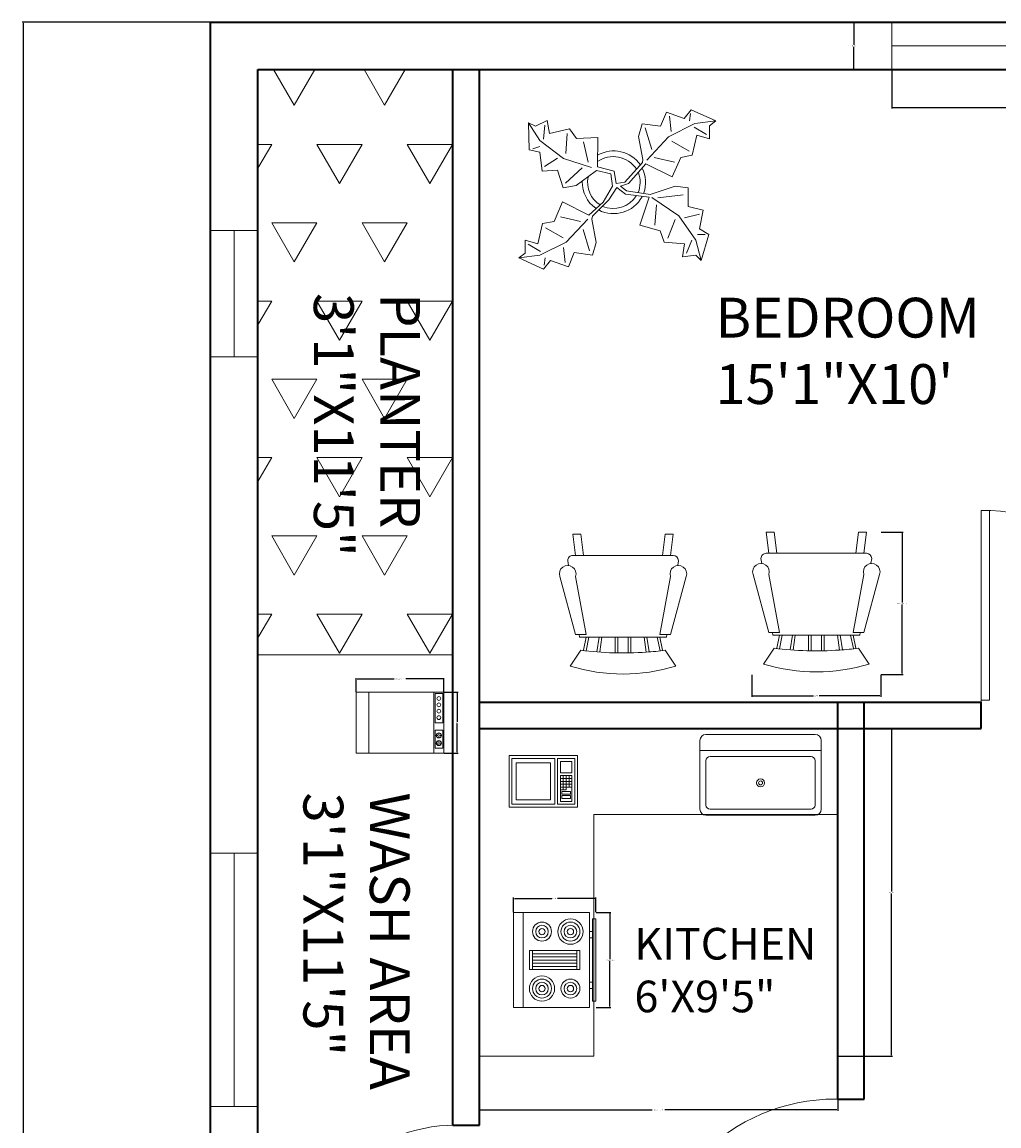
# Model space of a CAD drawing. Units: inches. Extents: x 7766 to 8631, y 9203 to 9940.
# Tile 3 of 6: x 7766 to 7952, y 9695 to 9905. Entities that reach past the tile are written whole.
import ezdxf

# ---------------------------------------------------------------- set-up
doc = ezdxf.new("R2010")
doc.units = ezdxf.units.IN
for name, color, linetype, lineweight in [('A-ANNO-DIMS', 2, 'Continuous', 18), ('A-AREA-IDEN', 11, 'Continuous', 18), ('A-EQPM', 9, 'Continuous', 18), ('A-FLOR-CASE', 7, 'Continuous', 20), ('A-FLOR-FIXT', 9, 'Continuous', 18), ('A-WALL', 7, 'Continuous', 35), ('door', 1, 'Continuous', 18), ('flower', 70, 'Continuous', 18), ('furniture', 6, 'Continuous', 18), ('L-PLNT-PATT', 60, 'Continuous', 13), ('window', 3, 'Continuous', 18)]:
    doc.layers.add(name, color=color, linetype=linetype, lineweight=lineweight)
doc.styles.get("Standard").update_dxf_attribs({"font": 'arial.ttf'})
doc.dimstyles.get("Standard").update_dxf_attribs({"dimtxt": 0.18, "dimasz": 0.18, "dimexe": 0.18, "dimexo": 0.0625, "dimgap": 0.09, "dimtad": 0, "dimtih": 1, "dimtoh": 1, "dimdec": 4, "dimzin": 0, "dimdsep": 46, "dimtxsty": 'Standard', "dimcen": 0.09, "dimadec": 0, "dimazin": 0, "dimtfac": 1, "dimtdec": 4, "dimtofl": 0, "dimtmove": 0, "dimatfit": 3, "dimfxl": 1, "dimtolj": 1, "dimtzin": 0, "dimarcsym": 0})

# ---------------------------------------------------------------- blocks, each defined once
blk = doc.blocks.new('*U2')
for p, q in [((0, 0), (0, -6)), ((40, 0), (40, -6))]:
    blk.add_line(p, q)
blk.add_lwpolyline([(0, 0), (0, 40), (1.75, 40), (1.75, 0)], close=True)
blk.add_arc((0, 0), 40, 0, 90)
blk = doc.blocks.new('*U4')
for p, q in [((0, 0), (0, -6)), ((40, 0), (40, -6))]:
    blk.add_line(p, q)
blk.add_lwpolyline([(0, 0), (0, 40), (1.75, 40), (1.75, 0)], close=True)
blk.add_arc((0, 0), 40, 0, 90)
blk = doc.blocks.new('Chair - Rocking')
for p, q in [((-8, -4.5), (-10, -1.5)), ((8, -4.5), (10, -1.5)), ((-4, -7), (-4.40532, -4.16272)), ((-1.5, -4.05012), (-1.5, -7)), ((-1, -7), (-1, -4.05012)), ((1, -7), (1, -4.04655)), ((1.5, -4.05012), (1.5, -7)), ((-7.5, -4.5), (-7, -7)), ((-6.5, -7), (-7.02225, -4.43)), ((-4.5, -7), (-4.96674, -4.19951)), ((4, -7), (4.40187, -4.18694)), ((4.5, -7), (4.96761, -4.19437)), ((6.5, -7), (7, -4.4057)), ((7.5, -4.5), (7, -7)), ((-9, -7.5), (-12, -18.49999)), ((-7, -7.5), (-9, -7.5)), ((-9, -18.49999), (-7, -7.5)), ((-8.23428, -6.99939), (-8.3093, -7.47958)), ((-8.23041, -7), (8.23915, -7)), ((7, -7.5), (9, -7.5)), ((9, -18.49999), (7, -7.5)), ((8.31071, -7.48854), (8.23449, -7.00073)), ((9, -7.5), (12, -18.49999)), ((-10.36644, -20.64523), (-10.5, -21.49999)), ((10.5, -21.49999), (10.3575, -20.58798)), ((-9, -22.49999), (-9.5, -26.49999)), ((0, -22.49999), (-9.5, -22.49999)), ((-8, -26.49999), (-7.5, -22.49999)), ((0, -22.49999), (9.5, -22.49999)), ((8, -26.49999), (7.5, -22.49999)), ((9, -22.49999), (9.5, -26.49999)), ((-9.5, -26.49999), (-8, -26.49999)), ((9.5, -26.49999), (8, -26.49999))]:
    blk.add_line(p, q)
for centre, radius, start, end in [((0, -34.08333), 34.08333, 72.93847, 107.0615), ((0, -68.25004), 64.25, 93.92211, 97.15267), ((0, -68.25004), 64.25, 82.84733, 93.92211), ((-10.5, -18.99999), 1.58114, 161.5651, 18.43495), ((10.5, -18.99999), 1.58114, 161.5651, 18.43495), ((-9.5, -21.49999), 1, 180, 270), ((9.5, -21.49999), 1, 270, 0)]:
    blk.add_arc(centre, radius, start, end)
blk = doc.blocks.new('Microwave')
for p, q in [((18, 10), (22, 10)), ((22, 9), (18, 9)), ((18, 8), (22, 8)), ((19, 7), (19, 11)), ((20, 11), (20, 7)), ((21, 7), (21, 11)), ((22, 7), (18, 7)), ((20, 6), (18, 6)), ((19, 6), (19, 7)), ((20, 7), (20, 6))]:
    blk.add_line(p, q)
for points in [[(0, 0), (0, 18), (24, 18), (24, 0)], [(1, 1), (1, 17), (16, 17), (16, 1)], [(2.5, 2.5), (2.5, 15.5), (14.5, 15.5), (14.5, 2.5)], [(17, 1), (17, 17), (23, 17), (23, 1)], [(18, 12), (18, 16), (22, 16), (22, 12)], [(18, 2), (18, 11), (22, 11), (22, 2)], [(18.5, 4.5), (18.5, 5.5), (21.5, 5.5), (21.5, 4.5)], [(18.5, 3), (18.5, 4), (21.5, 4), (21.5, 3)]]:
    blk.add_lwpolyline(points, close=True)
blk = doc.blocks.new('Range-Oven - 30 in top')
for p, q in [((0, -3), (30, -3)), ((12, -6), (18, -6)), ((13, -20), (13, -6)), ((14, -6), (14, -20)), ((15, -20), (15, -6)), ((16, -6), (16, -20)), ((17, -20), (17, -6)), ((18, -20), (12, -20)), ((6, -24), (6, -25)), ((8, -25), (8, -24)), ((22, -25), (22, -24)), ((24, -24), (24, -25))]:
    blk.add_line(p, q)
for points in [[(0, -24), (0, 0), (30, 0), (30, -24)], [(12, -21), (12, -5), (18, -5), (18, -21)], [(2, -26), (2, -25), (28, -25), (28, -26)]]:
    blk.add_lwpolyline(points, close=True)
for centre, radius in [((6, -9), 4), ((6, -9), 3), ((24, -9), 3), ((6, -9), 2), ((6, -9), 1), ((24, -9), 2), ((24, -9), 1), ((6, -18), 3), ((6, -18), 2), ((6, -18), 1), ((24, -18), 4), ((24, -18), 3), ((24, -18), 2), ((24, -18), 1)]:
    blk.add_circle(centre, radius)
blk = doc.blocks.new('Sink-single - 30 in top')
blk.add_line((-15, -3.999996), (15, -3.999996))
for points in [[(-13.5, 0), (13.5, 0)], [(-15, -18.499996), (-15, -1.5)], [(15, -1.5), (15, -18.499996)], [(-13.5, -17.499996), (-13.5, -6.499996)], [(-12.5, -5.499996), (12.5, -5.499996)], [(13.5, -6.499996), (13.5, -17.499996)], [(12.5, -18.499996), (-12.5, -18.499996)], [(13.5, -19.999996), (-13.5, -19.999996)]]:
    blk.add_lwpolyline(points)
for radius in [1, 0.5]:
    blk.add_circle((0, -11.999996), radius)
for centre, radius, start, end in [((-13.5, -1.5), 1.5, 90, 180), ((13.5, -1.5), 1.5, 0, 90), ((-12.5, -6.499996), 1, 90, 180), ((12.5, -6.499996), 1, 0, 90), ((-13.5, -18.499996), 1.5, 180, 270), ((-12.5, -17.499996), 1, 180, 270), ((12.5, -17.499996), 1, 270, 0), ((13.5, -18.499996), 1.5, 270, 0)]:
    blk.add_arc(centre, radius, start, end)
blk = doc.blocks.new('Plant - Rubber or Philodendron')
for p, q in [((8.8871, 10.7908), (9.9809, 13.4933)), ((9.9809, 13.4933), (13.3837, 12.301)), ((10.5828, 12.6946), (10.8893, 9.7953)), ((13.3837, 12.301), (14.68, 13.9039)), ((14.5816, 13.2037), (14.3848, 11.8033)), ((14.68, 13.9039), (19.3848, 11.8146)), ((-16.2005, 11.4774), (-13.9899, 8.1064)), ((-16.2005, 11.4774), (-14.8639, 10.7964)), ((-16.0159, 6.3329), (-16.2005, 11.4774)), ((-14.8639, 10.7964), (-12.6195, 11.8975)), ((-13.3174, 8.325), (-13.0735, 11.0065)), ((-12.6195, 11.8975), (-12.1909, 9.4345)), ((4.6914, 8.8812), (5.3859, 11.2828)), ((5.3859, 11.2828), (8.8871, 10.7908)), ((5.9878, 10.4842), (7.1971, 6.3869)), ((15.3859, 11.3055), (10.3916, 8.7942)), ((15.2875, 10.6053), (17.5907, 9.2105)), ((19.3848, 11.8146), (15.3859, 11.3055)), ((19.3848, 11.8146), (18.1868, 10.9119)), ((18.1868, 10.9119), (18.1925, 8.4119)), ((-12.1909, 9.4345), (-8.3829, 10.3)), ((-8.8369, 9.409), (-9.0894, 5.6095)), ((-8.3829, 10.3), (-7.0549, 8.501)), ((-7.0549, 8.501), (-3.0284, 8.6941)), ((-3.0284, 8.6941), (-3.0709, 3.1041)), ((4.6914, 8.8812), (5.5014, 4.4831)), ((10.3916, 8.7942), (6.2847, 4.4028)), ((15.7909, 9.1065), (14.8995, 5.3044)), ((18.1925, 8.4119), (15.7909, 9.1065)), ((-14.0069, 5.8704), (-16.0159, 6.3329)), ((-15.3434, 6.5514), (-13.9984, 6.9884)), ((-13.9899, 8.1064), (-9.5434, 4.7185)), ((-4.8529, 4.012), (-5.7184, 7.82)), ((14.2977, 6.1031), (10.9934, 7.9956)), ((-13.5868, 2.2894), (-14.0069, 5.8704)), ((-13.1329, 3.1804), (-10.6614, 4.727)), ((-9.5434, 4.7185), (-4.1917, 2.9888)), ((5.4346, 3.9146), (5.5014, 4.4831)), ((7.7005, 4.8881), (11.5025, 3.9967)), ((12.7005, 4.8994), (11.1089, 1.1958)), ((14.8995, 5.3044), (12.7005, 4.8994)), ((-10.6784, 2.491), (-13.5868, 2.2894)), ((-9.5858, -0.8715), (-10.6784, 2.491)), ((-9.1318, 0.0195), (-5.9793, 2.9025)), ((-7.1228, -0.443), (-3.5248, 2.2131)), ((-3.5248, 2.2131), (-3.3011, 2.4355)), ((-3.3011, 2.4355), (-0.5306, 1.7947)), ((-3.0709, 3.1041), (0.0797, 2.3163)), ((0.0797, 2.3163), (0.4866, -0.031)), ((2.1141, 0.2298), (5.4346, 3.9146)), ((6.1032, 3.6844), (2.8262, -0.031)), ((11.1089, 1.1958), (6.1032, 3.6844)), ((-0.5306, 1.7947), (-0.2255, -0.5527)), ((-0.5306, 1.7947), (-0.5306, 1.7947)), ((0.4866, -0.031), (2.1141, 0.2298)), ((-7.1228, -0.443), (-9.5858, -0.8715)), ((-2.019, -3.6148), (-0.2255, -0.5527)), ((-0.9375, -3.1608), (0.5883, -0.8135)), ((0.5883, -0.8135), (2.2447, -2.0916)), ((2.8262, -0.031), (1.3003, -0.5527)), ((1.3003, -0.5527), (2.4193, -1.4655)), ((2.2447, -2.0916), (6.7108, -2.6626)), ((2.4193, -1.4655), (6.895, -2.1175)), ((11.6605, -0.5413), (6.895, -2.1175)), ((11.6605, -0.5413), (14.1354, -0.8948)), ((14.1354, -0.8948), (14.1354, -4.4304)), ((-11.3237, -7.2629), (-9.7321, -3.5593)), ((-9.7321, -3.5593), (-4.7264, -6.0479)), ((-2.019, -3.6148), (-4.7264, -6.0479)), ((-4.0579, -6.2781), (-0.9375, -3.1608)), ((4.943, -7.9659), (6.7108, -2.6626)), ((12.3677, -6.1981), (7.219, -2.6772)), ((8.125, -4.0768), (7.7715, -7.9659)), ((8.3544, -2.7453), (13.1973, -2.1704)), ((-4.1246, -6.8466), (-4.0579, -6.2781)), ((15.5496, -10.7943), (12.3677, -6.1981)), ((16.2567, -5.8446), (13.4283, -6.5517)), ((14.1354, -4.4304), (16.9638, -5.1375)), ((16.9638, -5.1375), (16.2567, -8.673)), ((-14.4141, -11.4699), (-13.5228, -7.6679)), ((-13.5228, -7.6679), (-11.3237, -7.2629)), ((-6.3237, -7.2516), (-10.1257, -6.3602)), ((-9.0148, -11.1577), (-4.9047, -6.8122)), ((-3.3146, -11.2447), (-4.1246, -6.8466)), ((8.8321, -9.0266), (4.943, -7.9659)), ((10.2463, -10.4408), (11.6605, -6.9053)), ((-12.921, -8.4665), (-9.6166, -10.359)), ((-4.611, -12.8477), (-5.8203, -8.7504)), ((9.5392, -11.1479), (8.8321, -9.0266)), ((17.3174, -9.7337), (15.9032, -9.7337)), ((16.2567, -8.673), (18.0245, -9.7337)), ((18.0245, -9.7337), (16.6103, -14.6834)), ((-16.8157, -10.7754), (-14.4141, -11.4699)), ((-16.8101, -13.2754), (-16.8157, -10.7754)), ((-13.9107, -12.9688), (-16.2139, -11.574)), ((-14.0091, -13.669), (-9.0148, -11.1577)), ((-9.206, -15.0581), (-9.5126, -12.1588)), ((-3.3146, -11.2447), (-4.0092, -13.6463)), ((13.4283, -11.5015), (9.5392, -11.1479)), ((13.0748, -13.9763), (13.4283, -11.5015)), ((14.8425, -10.7943), (13.7819, -13.2692)), ((16.6103, -14.6834), (15.5496, -10.7943)), ((-18.008, -14.1781), (-16.8101, -13.2754)), ((-18.008, -14.1781), (-14.0091, -13.669)), ((-13.3032, -16.2674), (-18.008, -14.1781)), ((-13.2048, -15.5672), (-13.008, -14.1668)), ((-7.5103, -13.1543), (-8.6042, -15.8568)), ((-4.0092, -13.6463), (-7.5103, -13.1543)), ((15.5496, -13.6228), (13.0748, -13.9763)), ((16.6103, -14.6834), (15.5496, -13.6228)), ((-12.0069, -14.6645), (-13.3032, -16.2674)), ((-8.6042, -15.8568), (-12.0069, -14.6645))]:
    blk.add_line(p, q)
for centre, radius, start, end in [((0, 0), 6.1275, 34.37569, 120.1028), ((-0.0601, -0.2075), 5.2461, 33.82192, 124.9414), ((-0.098, 0.1364), 6.1288, 341.2017, 26.09184), ((0.0308, 0.1664), 6, 178.6147, 235.1169), ((0.0308, 0.1664), 5, 168.1647, 238.6725), ((-0.2664, 0.1682), 5.2775, 338.4094, 20.03007), ((-0.0234, 0.3825), 6.1492, 242.5812, 331.2714), ((-0.1102, 0.4886), 5.2883, 247.3711, 327.472)]:
    blk.add_arc(centre, radius, start, end)
blk = doc.blocks.new('Dishwasher')
for p, q in [((24, 30.5), (0, 30.5)), ((16, 32.5), (16.75, 32.5)), ((16.5, 32), (16.2942, 31.7942)), ((16.3156, 33.1843), (16.5, 33)), ((17, 32.75), (17, 33.5)), ((17, 32.25), (17, 31.5)), ((18, 32.5), (17.25, 32.5)), ((17.5, 33), (17.6938, 33.1938)), ((17.7061, 31.7939), (17.5, 32)), ((19, 32.5), (19.75, 32.5)), ((19.5, 32), (19.2942, 31.7942)), ((19.3156, 33.1843), (19.5, 33)), ((20, 32.75), (20, 33.5)), ((20, 32.25), (20, 31.5)), ((21, 32.5), (20.25, 32.5)), ((20.5, 33), (20.6938, 33.1938)), ((20.7061, 31.7939), (20.5, 32)), ((0, 5), (24, 5))]:
    blk.add_line(p, q)
for points in [[(0, 0), (0, 34.5), (24, 34.5), (24, 0)], [(0.5, 31), (0.5, 34), (12, 34), (12, 31)], [(15, 31), (15, 34), (22, 34), (22, 31)]]:
    blk.add_lwpolyline(points, close=True)
for centre, radius in [((2.5, 32.5), 0.75), ((5, 32.5), 0.75), ((7.5, 32.5), 0.75), ((10, 32.5), 0.75), ((17, 32.5), 1), ((20, 32.5), 1)]:
    blk.add_circle(centre, radius)
blk = doc.blocks.new('WIN-48IN')
blk.add_line((4.5, 48), (4.5, 0))
blk.add_lwpolyline([(0, 48), (9, 48), (9, 0), (0, 0)], close=True)
blk = doc.blocks.new('WIN-24IN')
blk.add_line((4.5, 24), (4.5, 0))
blk.add_lwpolyline([(0, 24), (9, 24), (9, 0), (0, 0)], close=True)
blk = doc.blocks.new('COUNTER-L-KITCHEN')
for points in [[(21.71, 45.84), (68, 45.84), (68, 62.12), (0, 62.12), (0, 45.84)], [(21.71, 45.84), (21.71, 0), (0, 0), (0, 62.12), (21.71, 62.12)]]:
    blk.add_lwpolyline(points)
blk = doc.blocks.new('*D28')
at = {"layer": 'A-ANNO-DIMS', "color": 0, "lineweight": -2, "transparency": 16777216}
for p, q in [((7931.49, 9895.5), (7931.49, 9888.18)), ((7979.49, 9895.5), (7979.49, 9888.18)), ((7931.67, 9888.36), (7954.37, 9888.36)), ((7979.31, 9888.36), (7956.61, 9888.36))]:
    blk.add_line(p, q, dxfattribs=at)
at = {"layer": 'A-ANNO-DIMS', "color": 0, "transparency": 16777216}
for points in [[(7931.67, 9888.39), (7931.67, 9888.33), (7931.49, 9888.36)], [(7979.31, 9888.39), (7979.31, 9888.33), (7979.49, 9888.36)]]:
    blk.add_solid(points, dxfattribs=at)
at = {"layer": 'Defpoints', "color": 0, "transparency": 16777216}
for p in [(7931.49, 9895.56), (7979.49, 9895.56), (7931.49, 9888.36)]:
    blk.add_point(p, dxfattribs=at)
at = {"layer": 'A-ANNO-DIMS', "color": 0, "transparency": 16777216, "insert": (7955.49, 9888.36), "char_height": 0.18, "attachment_point": 5}
blk.add_mtext('\\A1;WINDOW 48 TYP.', dxfattribs=at)
blk = doc.blocks.new('*D29')
at = {"layer": 'A-ANNO-DIMS', "color": 0, "lineweight": -2, "transparency": 16777216}
for p, q in [((7931.43, 9904.56), (7924.11, 9904.56)), ((7924.29, 9904.38), (7924.29, 9900.25)), ((7924.29, 9895.74), (7924.29, 9899.88)), ((7931.43, 9895.56), (7924.11, 9895.56))]:
    blk.add_line(p, q, dxfattribs=at)
at = {"layer": 'A-ANNO-DIMS', "color": 0, "transparency": 16777216}
for points in [[(7924.26, 9904.38), (7924.32, 9904.38), (7924.29, 9904.56)], [(7924.26, 9895.74), (7924.32, 9895.74), (7924.29, 9895.56)]]:
    blk.add_solid(points, dxfattribs=at)
at = {"layer": 'Defpoints', "color": 0, "transparency": 16777216}
for p in [(7924.29, 9904.56), (7931.49, 9904.56), (7931.49, 9895.56)]:
    blk.add_point(p, dxfattribs=at)
at = {"layer": 'A-ANNO-DIMS', "color": 0, "transparency": 16777216, "insert": (7924.29, 9900.06), "char_height": 0.18, "attachment_point": 5}
blk.add_mtext('\\A1;9 TYP.', dxfattribs=at)
blk = doc.blocks.new('*D38')
at = {"layer": 'A-ANNO-DIMS', "color": 0, "lineweight": -2, "transparency": 16777216}
for p, q in [((7929.46, 9807.81), (7933.63, 9807.81)), ((7933.45, 9807.63), (7933.45, 9794.5)), ((7933.45, 9780.99), (7933.45, 9794.13)), ((7929.46, 9780.81), (7933.63, 9780.81))]:
    blk.add_line(p, q, dxfattribs=at)
at = {"layer": 'A-ANNO-DIMS', "color": 0, "transparency": 16777216}
for points in [[(7933.42, 9807.63), (7933.48, 9807.63), (7933.45, 9807.81)], [(7933.42, 9780.99), (7933.48, 9780.99), (7933.45, 9780.81)]]:
    blk.add_solid(points, dxfattribs=at)
at = {"layer": 'Defpoints', "color": 0, "transparency": 16777216}
for p in [(7929.4, 9807.81), (7929.4, 9780.81), (7933.45, 9780.81)]:
    blk.add_point(p, dxfattribs=at)
at = {"layer": 'A-ANNO-DIMS', "color": 0, "transparency": 16777216, "insert": (7933.45, 9794.31), "char_height": 0.18, "attachment_point": 5}
blk.add_mtext('\\A1;ROCKER 27 TYP.', dxfattribs=at)
blk = doc.blocks.new('*D39')
at = {"layer": 'A-ANNO-DIMS', "color": 0, "lineweight": -2, "transparency": 16777216}
for p, q in [((7904.96, 9780.75), (7904.96, 9776.58)), ((7929.4, 9780.75), (7929.4, 9776.58)), ((7905.14, 9776.76), (7916.65, 9776.76)), ((7929.22, 9776.76), (7917.71, 9776.76))]:
    blk.add_line(p, q, dxfattribs=at)
at = {"layer": 'A-ANNO-DIMS', "color": 0, "transparency": 16777216}
for points in [[(7905.14, 9776.79), (7905.14, 9776.73), (7904.96, 9776.76)], [(7929.22, 9776.79), (7929.22, 9776.73), (7929.4, 9776.76)]]:
    blk.add_solid(points, dxfattribs=at)
at = {"layer": 'Defpoints', "color": 0, "transparency": 16777216}
for p in [(7904.96, 9780.81), (7929.4, 9780.81), (7904.96, 9776.76)]:
    blk.add_point(p, dxfattribs=at)
at = {"layer": 'A-ANNO-DIMS', "color": 0, "transparency": 16777216, "insert": (7917.18, 9776.76), "char_height": 0.18, "attachment_point": 5}
blk.add_mtext('\\A1;24 TYP.', dxfattribs=at)
blk = doc.blocks.new('*D48')
at = {"layer": 'A-ANNO-DIMS', "color": 0, "lineweight": -2, "transparency": 16777216}
for p, q in [((7875.39, 9735.67), (7878.21, 9735.67)), ((7878.03, 9735.49), (7878.03, 9726.85)), ((7878.03, 9717.85), (7878.03, 9726.48)), ((7875.39, 9717.67), (7878.21, 9717.67))]:
    blk.add_line(p, q, dxfattribs=at)
at = {"layer": 'A-ANNO-DIMS', "color": 0, "transparency": 16777216}
for points in [[(7878, 9735.49), (7878.06, 9735.49), (7878.03, 9735.67)], [(7878, 9717.85), (7878.06, 9717.85), (7878.03, 9717.67)]]:
    blk.add_solid(points, dxfattribs=at)
at = {"layer": 'Defpoints', "color": 0, "transparency": 16777216}
for p in [(7875.33, 9735.67), (7878.03, 9735.67), (7875.33, 9717.67)]:
    blk.add_point(p, dxfattribs=at)
at = {"layer": 'A-ANNO-DIMS', "color": 0, "transparency": 16777216, "insert": (7878.03, 9726.67), "char_height": 0.18, "attachment_point": 5}
blk.add_mtext('\\A1;RANGE 18 TYP.', dxfattribs=at)
blk = doc.blocks.new('*D49')
at = {"layer": 'A-ANNO-DIMS', "color": 0, "lineweight": -2, "transparency": 16777216}
for p, q in [((7859.73, 9735.73), (7859.73, 9738.55)), ((7859.91, 9738.37), (7867.01, 9738.37)), ((7875.15, 9738.37), (7868.05, 9738.37)), ((7875.33, 9735.73), (7875.33, 9738.55))]:
    blk.add_line(p, q, dxfattribs=at)
at = {"layer": 'A-ANNO-DIMS', "color": 0, "transparency": 16777216}
for points in [[(7859.91, 9738.4), (7859.91, 9738.34), (7859.73, 9738.37)], [(7875.15, 9738.4), (7875.15, 9738.34), (7875.33, 9738.37)]]:
    blk.add_solid(points, dxfattribs=at)
at = {"layer": 'Defpoints', "color": 0, "transparency": 16777216}
for p in [(7859.73, 9738.37), (7859.73, 9735.67), (7875.33, 9735.67)]:
    blk.add_point(p, dxfattribs=at)
at = {"layer": 'A-ANNO-DIMS', "color": 0, "transparency": 16777216, "insert": (7867.53, 9738.37), "char_height": 0.18, "attachment_point": 5}
blk.add_mtext('\\A1;16 TYP.', dxfattribs=at)
blk = doc.blocks.new('*D62')
at = {"layer": 'A-ANNO-DIMS', "color": 0, "lineweight": -2, "transparency": 16777216}
for p, q in [((7853.24, 9708.38), (7853.24, 9698.06)), ((7921.24, 9708.38), (7921.24, 9698.06)), ((7853.42, 9698.24), (7886.06, 9698.24)), ((7921.06, 9698.24), (7888.43, 9698.24))]:
    blk.add_line(p, q, dxfattribs=at)
at = {"layer": 'A-ANNO-DIMS', "color": 0, "transparency": 16777216}
for points in [[(7853.42, 9698.27), (7853.42, 9698.21), (7853.24, 9698.24)], [(7921.06, 9698.27), (7921.06, 9698.21), (7921.24, 9698.24)]]:
    blk.add_solid(points, dxfattribs=at)
at = {"layer": 'Defpoints', "color": 0, "transparency": 16777216}
for p in [(7853.24, 9708.44), (7921.24, 9708.44), (7921.24, 9698.24)]:
    blk.add_point(p, dxfattribs=at)
at = {"layer": 'A-ANNO-DIMS', "color": 0, "transparency": 16777216, "insert": (7887.24, 9698.24), "char_height": 0.18, "attachment_point": 5}
blk.add_mtext('\\A1;COUNTER 68 TYP.', dxfattribs=at)
blk = doc.blocks.new('*D63')
at = {"layer": 'A-ANNO-DIMS', "color": 0, "lineweight": -2, "transparency": 16777216}
for p, q in [((7921.31, 9770.56), (7931.62, 9770.56)), ((7931.44, 9770.38), (7931.44, 9739.68)), ((7931.44, 9708.62), (7931.44, 9739.32)), ((7921.31, 9708.44), (7931.62, 9708.44))]:
    blk.add_line(p, q, dxfattribs=at)
at = {"layer": 'A-ANNO-DIMS', "color": 0, "transparency": 16777216}
for points in [[(7931.41, 9770.38), (7931.47, 9770.38), (7931.44, 9770.56)], [(7931.41, 9708.62), (7931.47, 9708.62), (7931.44, 9708.44)]]:
    blk.add_solid(points, dxfattribs=at)
at = {"layer": 'Defpoints', "color": 0, "transparency": 16777216}
for p in [(7921.24, 9770.56), (7931.44, 9770.56), (7921.24, 9708.44)]:
    blk.add_point(p, dxfattribs=at)
at = {"layer": 'A-ANNO-DIMS', "color": 0, "transparency": 16777216, "insert": (7931.44, 9739.5), "char_height": 0.18, "attachment_point": 5}
blk.add_mtext('\\A1;62 TYP.', dxfattribs=at)
blk = doc.blocks.new('*D66')
at = {"layer": 'A-ANNO-DIMS', "color": 0, "lineweight": -2, "transparency": 16777216}
for p, q in [((7829.87, 9777.55), (7829.87, 9780.16)), ((7830.05, 9779.98), (7837.1, 9779.98)), ((7846.35, 9779.98), (7839.3, 9779.98)), ((7846.53, 9777.55), (7846.53, 9780.16))]:
    blk.add_line(p, q, dxfattribs=at)
at = {"layer": 'A-ANNO-DIMS', "color": 0, "transparency": 16777216}
for points in [[(7830.05, 9780.01), (7830.05, 9779.95), (7829.87, 9779.98)], [(7846.35, 9780.01), (7846.35, 9779.95), (7846.53, 9779.98)]]:
    blk.add_solid(points, dxfattribs=at)
at = {"layer": 'Defpoints', "color": 0, "transparency": 16777216}
for p in [(7846.53, 9779.98), (7829.87, 9777.49), (7846.53, 9777.49)]:
    blk.add_point(p, dxfattribs=at)
at = {"layer": 'A-ANNO-DIMS', "color": 0, "transparency": 16777216, "insert": (7838.2, 9779.98), "char_height": 0.18, "attachment_point": 5}
blk.add_mtext('\\A1;DISHWASHER 17', dxfattribs=at)
blk = doc.blocks.new('*D67')
at = {"layer": 'A-ANNO-DIMS', "color": 0, "lineweight": -2, "transparency": 16777216}
for p, q in [((7846.59, 9777.49), (7849.21, 9777.49)), ((7849.03, 9777.31), (7849.03, 9771.87)), ((7849.03, 9766.08), (7849.03, 9771.51)), ((7846.59, 9765.9), (7849.21, 9765.9))]:
    blk.add_line(p, q, dxfattribs=at)
at = {"layer": 'A-ANNO-DIMS', "color": 0, "transparency": 16777216}
for points in [[(7849, 9777.31), (7849.06, 9777.31), (7849.03, 9777.49)], [(7849, 9766.08), (7849.06, 9766.08), (7849.03, 9765.9)]]:
    blk.add_solid(points, dxfattribs=at)
at = {"layer": 'Defpoints', "color": 0, "transparency": 16777216}
for p in [(7846.53, 9777.49), (7846.53, 9765.9), (7849.03, 9765.9)]:
    blk.add_point(p, dxfattribs=at)
at = {"layer": 'A-ANNO-DIMS', "color": 0, "transparency": 16777216, "insert": (7849.03, 9771.69), "char_height": 0.18, "attachment_point": 5}
blk.add_mtext('\\A1;12', dxfattribs=at)
blk = doc.blocks.new('*D69')
at = {"layer": 'A-ANNO-DIMS', "color": 0, "lineweight": -2, "transparency": 16777216}
for p, q in [((7802.18, 9904.56), (7766.51, 9904.56)), ((7766.69, 9904.38), (7766.69, 9600.25)), ((7766.69, 9295.74), (7766.69, 9599.88)), ((7802.18, 9295.56), (7766.51, 9295.56))]:
    blk.add_line(p, q, dxfattribs=at)
at = {"layer": 'A-ANNO-DIMS', "color": 0, "transparency": 16777216}
for points in [[(7766.66, 9904.38), (7766.72, 9904.38), (7766.69, 9904.56)], [(7766.66, 9295.74), (7766.72, 9295.74), (7766.69, 9295.56)]]:
    blk.add_solid(points, dxfattribs=at)
at = {"layer": 'Defpoints', "color": 0, "transparency": 16777216}
for p in [(7766.69, 9904.56), (7802.24, 9904.56), (7802.24, 9295.56)]:
    blk.add_point(p, dxfattribs=at)
at = {"layer": 'A-ANNO-DIMS', "color": 0, "transparency": 16777216, "insert": (7766.69, 9600.06), "char_height": 0.18, "attachment_point": 5}
blk.add_mtext('\\A1;609', dxfattribs=at)

msp = doc.modelspace()

# ---------------------------------------------------------------- hatches: boundary and pattern name
at = {"layer": 'L-PLNT-PATT'}
h = msp.add_hatch(dxfattribs=at)
h.set_pattern_fill('TRIANG', color=256, scale=1.8)
h.paths.add_polyline_path([(7848.243, 9895.5631), (7811.243, 9895.5631), (7811.243, 9784.5631), (7848.243, 9784.5631)])
h.paths.add_polyline_path([(7848.243, 9655.5631), (7811.243, 9655.5631), (7811.243, 9509.5631), (7848.243, 9509.5631)])
h.paths.add_polyline_path([(8058.243, 9372.5631), (7939.243, 9372.5631), (7939.243, 9304.5631), (8058.243, 9304.5631)])
h.paths.add_polyline_path([(7817.6934, 9855.8718), (7817.6934, 9803.4053), (7845.8896, 9803.4053), (7845.8896, 9855.8718)], flags=24)
h.paths.add_polyline_path([(7814.5059, 9594.625), (7814.5059, 9542.1584), (7842.7021, 9542.1584), (7842.7021, 9594.625)], flags=24)
h.paths.add_polyline_path([(7965.0141, 9329.808), (8013.9551, 9329.808), (8013.9551, 9358.0042), (7965.0141, 9358.0042)], flags=24)

# ---------------------------------------------------------------- linework, layer by layer
at = {"layer": 'A-WALL'}
for p, q in [((7802.243, 9295.5631), (7802.243, 9904.5631)), ((7802.243, 9904.5631), (8067.243, 9904.5631)), ((7811.243, 9509.5631), (7811.243, 9895.5631)), ((7811.243, 9895.5631), (8058.243, 9895.5631)), ((7848.243, 9695.3613), (7848.243, 9895.5631)), ((7853.243, 9695.3613), (7853.243, 9895.5631)), ((7853.243, 9775.5631), (7948.4542, 9775.5631)), ((7921.243, 9700.3108), (7921.243, 9775.5631)), ((7926.243, 9700.3108), (7926.243, 9775.5631)), ((7853.243, 9770.5631), (7948.4542, 9770.5631))]:
    msp.add_line(p, q, dxfattribs=at)
for points in [[(7948.4542, 9770.5631), (7948.4542, 9775.5631)], [(7921.243, 9700.3108), (7926.243, 9700.3108)], [(7848.243, 9695.3613), (7853.243, 9695.3613)]]:
    msp.add_lwpolyline(points, dxfattribs=at)
at = {"layer": 'flower'}
msp.add_line((7811.243, 9784.5631), (7848.243, 9784.5631), dxfattribs=at)
msp.add_lwpolyline([(7811.243, 9895.5631), (7848.243, 9895.5631), (7848.243, 9784.5631), (7811.243, 9784.5631)], close=True, dxfattribs=at)

# ---------------------------------------------------------------- block references
at = {"layer": 'A-EQPM'}
for name, p, xscale, yscale, zscale, rotation in [('Dishwasher', (7829.873, 9777.4858), 0.4828660506709771, 0.4828660506709771, 0.4828660506709771, 270), ('Range-Oven - 30 in top', (7859.7306, 9717.6671), 0.5999998666666216, 0.5999998666666216, 0.5999998666666216, 90)]:
    msp.add_blockref(name, p, dxfattribs=dict(at, xscale=xscale, yscale=yscale, zscale=zscale, rotation=rotation))
at = {"layer": 'A-EQPM', "xscale": 0.5416666666666666, "yscale": 0.5416666666666666, "zscale": 0.5416666666666666}
msp.add_blockref('Microwave', (7858.885, 9755.6895), dxfattribs=at)
at = {"layer": 'A-FLOR-CASE'}
msp.add_blockref('COUNTER-L-KITCHEN', (7853.243, 9708.441), dxfattribs=at)
at = {"layer": 'A-FLOR-FIXT', "xscale": 0.7668297541752571, "yscale": 0.7668297541752571, "zscale": 0.7668297541752571}
msp.add_blockref('Sink-single - 30 in top', (7906.5947, 9769.4766), dxfattribs=at)
at = {"layer": 'door', "xscale": 0.9, "yscale": 0.9, "zscale": 0.9}
msp.add_blockref('*U2', (7948.4542, 9775.9631), dxfattribs=at)
at = {"layer": 'door', "rotation": 90}
for name, p, xscale, yscale, zscale in [('*U4', (7920.843, 9664.3108), 0.9, 0.9, 0.9), ('*U2', (7848.743, 9665.3613), 0.75, 0.75, 0.75)]:
    msp.add_blockref(name, p, dxfattribs=dict(at, xscale=xscale, yscale=yscale, zscale=zscale))
at = {"layer": 'flower'}
msp.add_blockref('Plant - Rubber or Philodendron', (7878.7401, 9874.0011), dxfattribs=at)
at = {"layer": 'furniture', "rotation": 180}
for p in [(7917.1792, 9781.3146), (7880.504, 9780.9193)]:
    msp.add_blockref('Chair - Rocking', p, dxfattribs=at)
at = {"layer": 'window', "rotation": 89.99999999999748}
msp.add_blockref('WIN-48IN', (7979.4895, 9895.5631), dxfattribs=at)
at = {"layer": 'window'}
for name, p in [('WIN-24IN', (7802.243, 9841.0512)), ('WIN-48IN', (7802.243, 9698.921))]:
    msp.add_blockref(name, p, dxfattribs=at)

# ---------------------------------------------------------------- texts
at = {"layer": 'A-AREA-IDEN', "char_height": 7.55634, "attachment_point": 1, "rotation": 270}
for s, insert in [('PLANTER\\P3\'1"X11\'5"', (7842.0007, 9853.1684)), ('WASH AREA\\P3\'1"X11\'5"', (7840.025, 9758.456))]:
    msp.add_mtext_dynamic_manual_height_columns(s, width=97.347002, gutter_width=18.8909, heights=[0], dxfattribs=dict(at, insert=insert))
at = {"layer": 'A-AREA-IDEN', "attachment_point": 1}
for s, insert, char_height in [('BEDROOM \\P15\'1"X10\'', (7898.0403, 9852.2835), 7.55634), ('KITCHEN\\P6\'X9\'5"', (7882.6666, 9732.7702), 6)]:
    msp.add_mtext_dynamic_manual_height_columns(s, width=97.347002, gutter_width=18.8909, heights=[0], dxfattribs=dict(at, insert=insert, char_height=char_height))

# ---------------------------------------------------------------- dimensions: what is measured, and where the dimension line sits
at = {"layer": 'A-ANNO-DIMS'}
for base, p1, p2, angle, picture, middle in [((7766.693, 9904.5631), (7802.243, 9295.5631), (7802.243, 9904.5631), 90, '*D69', (7766.693, 9600.0631)), ((7849.0308, 9765.897), (7846.5319, 9777.4858), (7846.5319, 9765.897), 270, '*D67', (7849.0308, 9771.6914))]:
    dim = msp.add_linear_dim(base=base, p1=p1, p2=p2, angle=angle, dimstyle='Standard', override={"dimdec": 0, "dimlfac": 1, "dimrnd": 0, "dimzin": 0, "dimdsep": 46, "dimlunit": 2}, dxfattribs=at)
    dim.commit()
    dim.dimension.update_dxf_attribs({"geometry": picture, "text_midpoint": middle})
for base, p1, p2, angle, text, picture, middle in [((7924.2899, 9904.5631), (7931.4899, 9895.5631), (7931.4899, 9904.5631), 90, '<> TYP.', '*D29', (7924.2899, 9900.0631)), ((7931.4899, 9888.3631), (7979.4899, 9895.5631), (7931.4899, 9895.5631), 180, 'WINDOW <> TYP.', '*D28', (7955.4899, 9888.3631)), ((7933.4468, 9780.8146), (7929.3968, 9807.8145), (7929.3968, 9780.8146), 270, 'ROCKER <> TYP.', '*D38', (7933.4468, 9794.3145)), ((7904.9617, 9776.7646), (7929.3968, 9780.8146), (7904.9617, 9780.8146), 180, '<> TYP.', '*D39', (7917.1792, 9776.7646)), ((7931.443, 9770.5631), (7921.243, 9708.4413), (7921.243, 9770.5631), 90, '<> TYP.', '*D63', (7931.443, 9739.5022)), ((7859.7306, 9738.3671), (7875.3306, 9735.6671), (7859.7306, 9735.6671), 180, '<> TYP.', '*D49', (7867.5306, 9738.3671)), ((7878.0306, 9735.6671), (7875.3306, 9717.6671), (7875.3306, 9735.6671), 90, 'RANGE <> TYP.', '*D48', (7878.0306, 9726.6671))]:
    dim = msp.add_linear_dim(base=base, p1=p1, p2=p2, angle=angle, text=text, dimstyle='Standard', override={"dimdec": 0, "dimlfac": 1, "dimrnd": 0, "dimzin": 0, "dimdsep": 46, "dimlunit": 2}, dxfattribs=at)
    dim.commit()
    dim.dimension.update_dxf_attribs({"geometry": picture, "text_midpoint": middle})
for base, p1, p2, text, picture, middle in [((7846.5319, 9779.9846), (7829.873, 9777.4858), (7846.5319, 9777.4858), 'DISHWASHER <>', '*D66', (7838.2025, 9779.9846)), ((7921.243, 9698.2413), (7853.243, 9708.4413), (7921.243, 9708.4413), 'COUNTER <> TYP.', '*D62', (7887.243, 9698.2413))]:
    dim = msp.add_linear_dim(base=base, p1=p1, p2=p2, text=text, dimstyle='Standard', override={"dimdec": 0, "dimlfac": 1, "dimrnd": 0, "dimzin": 0, "dimdsep": 46, "dimlunit": 2}, dxfattribs=at)
    dim.commit()
    dim.dimension.update_dxf_attribs({"geometry": picture, "text_midpoint": middle})

doc.saveas('drawing.dxf')
